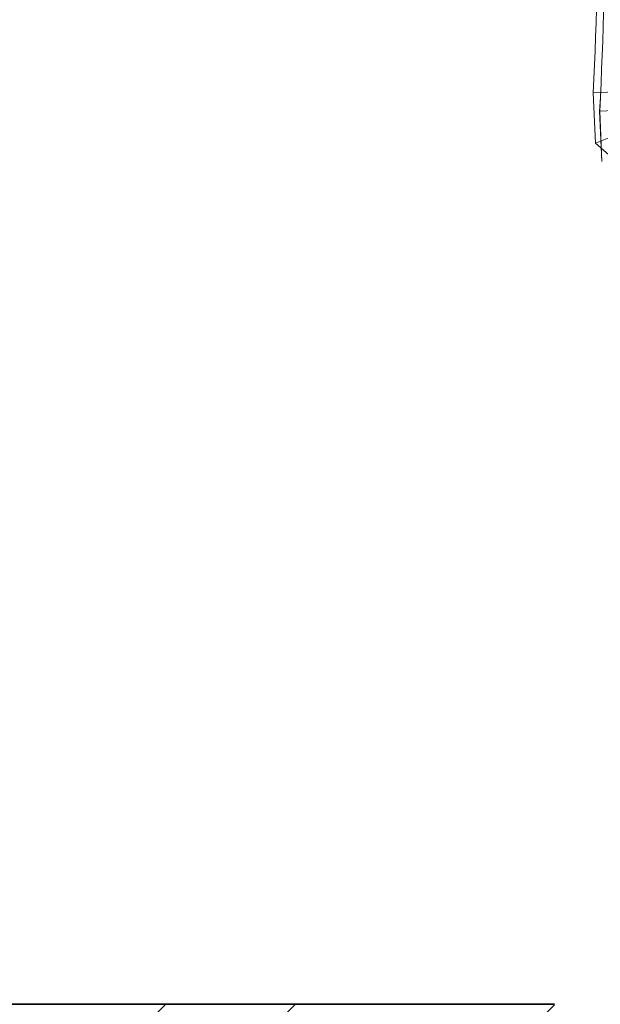
# Model space of a CAD drawing. Units: inches. Extents: x 1885 to 2748, y 783 to 2421.
# Tile 60 of 117: x 2029 to 2049, y 1886 to 1920. Entities that reach past the tile are written whole.
import ezdxf

# ---------------------------------------------------------------- set-up
doc = ezdxf.new("R2010")
doc.units = ezdxf.units.IN
doc.layers.add('A-FURN', color=8, linetype='Continuous', lineweight=13)
doc.layers.add('A-WALL', color=7, linetype='Continuous', lineweight=35)
doc.layers.add('A-WALL-PATT', color=85, linetype='Continuous', lineweight=13, true_color=0x58ba48)

# ---------------------------------------------------------------- blocks, each defined once
blk = doc.blocks.new('BED-DOUBLE')
for p, q in [((30.133, 53.174), (28.389, 53.095, 3.871)), ((30.133, 53.174), (28.389, 53.094, 3.871)), ((28.389, 53.095), (25.139, 49.389)), ((28.389, 53.094), (25.139, 49.389)), ((29.494, 52.946), (27.749, 52.866, 3.871)), ((29.494, 52.945), (27.75, 52.866, 3.871)), ((29.008, 51.558), (28.389, 53.095)), ((29.008, 51.557), (28.389, 53.094))]:
    blk.add_line(p, q)
for centre, radius, start, end in [((-6.013, 51.554), 36.183, 349.8763, 2.5657), ((-6.013, 51.554), 36.183, 349.8763, 2.5657), ((36.958, 182.493), 129.499, 266.97912, 273.83645), ((36.958, 182.493), 129.499, 266.97912, 273.83645), ((-6.653, 51.326), 36.183, 349.8763, 2.5657), ((-6.653, 51.326), 36.183, 349.8763, 2.5657), ((36.319, 182.265), 129.499, 266.97912, 273.83645), ((36.319, 182.264), 129.499, 266.97912, 273.83645)]:
    blk.add_arc(centre, radius, start, end)

msp = doc.modelspace()

# ---------------------------------------------------------------- hatches: boundary and pattern name
at = {"layer": 'A-WALL-PATT'}
h = msp.add_hatch(dxfattribs=at)
h.set_pattern_fill('ANSI32', color=256)
h.paths.add_polyline_path([(2007.772, 2318.006), (1980.774, 2318.006), (1980.774, 2281.215), (1985.274, 2281.215), (1985.274, 2313.506), (2007.772, 2313.506), (2007.772, 2315.756)])
h.paths.add_polyline_path([(2094.324, 2318.006), (2067.772, 2318.006), (2067.772, 2313.506), (2094.324, 2313.506), (2094.324, 2315.756)])
h.paths.add_polyline_path([(2131.367, 2315.756), (2131.367, 2318.006), (2131.189, 2318.006), (2112.609, 2318.006), (2112.609, 2313.506), (2117.274, 2313.506), (2117.274, 2255.201), (2121.774, 2255.201), (2121.774, 2313.506), (2131.367, 2313.506)])
h.paths.add_polyline_path([(2190.512, 2318.006), (2155.367, 2318.006), (2155.367, 2313.506), (2169.774, 2313.506), (2169.774, 2229.506), (2121.774, 2229.506), (2121.774, 2233.451), (2119.524, 2233.451), (2117.274, 2233.451), (2117.274, 2201.101), (2121.774, 2201.101), (2121.774, 2225.006), (2169.774, 2225.006), (2169.774, 2165.006), (2306.274, 2165.006), (2306.274, 2066.006), (2310.774, 2066.006), (2344.274, 2066.006), (2486.274, 2066.006), (2486.274, 1886.006), (2483.02, 1886.006), (2483.02, 1881.506), (2486.274, 1881.506), (2486.274, 1880.678), (2490.774, 1880.678), (2490.774, 2070.506), (2344.274, 2070.506), (2310.774, 2070.506), (2310.774, 2165.006), (2310.774, 2173.636), (2308.524, 2173.636), (2306.274, 2173.636), (2306.274, 2169.506), (2174.274, 2169.506), (2174.274, 2313.506), (2190.512, 2313.506), (2190.512, 2315.756)])
h.paths.add_polyline_path([(1985.274, 2221.215), (1980.774, 2221.215), (1980.774, 2165.006), (1992.774, 2165.006), (1992.774, 2141.927), (1997.274, 2141.927), (1997.274, 2165.006), (2117.274, 2165.006), (2117.274, 2163.126), (2121.774, 2163.126), (2121.774, 2172.734), (2119.524, 2172.734), (2117.274, 2172.734), (2117.274, 2169.506), (1985.274, 2169.506)])
h.paths.add_polyline_path([(1997.274, 2105.927), (1992.774, 2105.927), (1992.774, 2070.506), (2016.774, 2070.506), (2016.774, 2059.123), (2019.024, 2059.123), (2021.274, 2059.123), (2021.274, 2070.506), (2117.274, 2070.506), (2117.274, 2022.506), (2114.423, 2022.506), (2114.423, 2018.006), (2123.627, 2018.006), (2123.627, 2020.256), (2123.627, 2022.506), (2121.774, 2022.506), (2121.774, 2142.587), (2119.524, 2142.587), (2117.274, 2142.587), (2117.274, 2075.006), (1997.274, 2075.006)])
h.paths.add_polyline_path([(2092.029, 2020.256), (2092.029, 2022.506), (2021.274, 2022.506), (2021.274, 2035.123), (2016.774, 2035.123), (2016.774, 2018.006), (2016.774, 1978.784), (2021.274, 1978.784), (2021.274, 2018.006), (2092.029, 2018.006)])
h.paths.add_polyline_path([(2260.938, 2022.506), (2153.105, 2022.506), (2153.105, 2020.256), (2153.105, 2018.006), (2155.274, 2018.006), (2155.274, 1886.006), (2107.629, 1886.006), (2107.629, 1881.506), (2182.911, 1881.506), (2182.911, 1883.756), (2182.911, 1886.006), (2159.774, 1886.006), (2159.774, 2018.006), (2260.938, 2018.006), (2260.938, 2020.256)])
h.paths.add_polyline_path([(2047.629, 1883.756), (2047.629, 1886.006), (2021.274, 1886.006), (2021.274, 1918.784), (2019.024, 1918.784), (2016.774, 1918.784), (2016.774, 1881.506), (2047.629, 1881.506)])
h.paths.add_polyline_path([(2306.361, 1883.756), (2306.361, 1886.006), (2296.274, 1886.006), (2296.274, 1982.006), (2316.535, 1982.006), (2316.535, 1984.256), (2316.535, 1986.506), (2296.274, 1986.506), (2296.274, 2022.506), (2289.276, 2022.506), (2289.276, 2018.006), (2291.774, 2018.006), (2291.774, 1886.006), (2242.911, 1886.006), (2242.911, 1881.506), (2306.361, 1881.506)], flags=17)
h.paths.add_polyline_path([(1985.274, 1843.006), (2021.6, 1843.006), (2021.534, 1845.441), (2021.477, 1847.506), (1980.774, 1847.506), (1980.774, 1809.446), (1985.274, 1809.446)])
h.paths.add_polyline_path([(2131.482, 1845.256), (2131.482, 1847.506), (2081.534, 1847.506), (2081.534, 1843.006), (2117.274, 1843.006), (2117.274, 1784.147), (2119.524, 1784.147), (2121.774, 1784.147), (2121.774, 1843.006), (2131.482, 1843.006)])
h.paths.add_polyline_path([(2203.886, 1847.506), (2155.482, 1847.506), (2155.482, 1843.006), (2169.774, 1843.006), (2169.774, 1759.006), (2121.774, 1759.006), (2121.774, 1761.457), (2117.274, 1761.457), (2117.274, 1730.429), (2121.774, 1730.429), (2121.774, 1754.506), (2177.421, 1754.506), (2177.421, 1756.756), (2177.421, 1759.006), (2174.274, 1759.006), (2174.274, 1843.006), (2203.886, 1843.006)])
h.paths.add_polyline_path([(2335.554, 1845.256), (2335.554, 1847.506), (2239.886, 1847.506), (2239.886, 1843.006), (2306.274, 1843.006), (2306.274, 1759.006), (2199.486, 1759.006), (2199.486, 1754.506), (2310.774, 1754.506), (2310.774, 1843.006), (2335.554, 1843.006)])
h.paths.add_polyline_path([(2348.774, 2022.506), (2344.274, 2022.506), (2344.274, 1986.506), (2341.681, 1986.506), (2341.681, 1982.006), (2344.274, 1982.006), (2344.274, 1886.006), (2330.361, 1886.006), (2330.361, 1881.506), (2361.627, 1881.506), (2361.627, 1883.756), (2361.627, 1886.006), (2348.774, 1886.006)], flags=17)
h.paths.add_polyline_path([(2283.251, 2315.756), (2283.251, 2318.006), (2238.512, 2318.006), (2238.512, 2313.506), (2283.251, 2313.506)], flags=17)
h.paths.add_polyline_path([(2363.274, 2348.006), (2388.677, 2348.006), (2388.677, 2350.256), (2388.677, 2352.506), (2358.774, 2352.506), (2358.774, 2348.006), (2358.774, 2318.006), (2344.481, 2318.006), (2344.481, 2313.506), (2358.774, 2313.506), (2358.774, 2229.506), (2310.774, 2229.506), (2310.774, 2231.952), (2306.274, 2231.952), (2306.274, 2205.611), (2310.774, 2205.611), (2310.774, 2225.006), (2358.774, 2225.006), (2358.774, 2211.506), (2452.329, 2211.506), (2452.329, 2213.756), (2452.329, 2216.006), (2363.274, 2216.006), (2363.274, 2318.006)])
h.paths.add_polyline_path([(2310.774, 2313.506), (2320.481, 2313.506), (2320.481, 2315.756), (2320.481, 2318.006), (2302.728, 2318.006), (2302.728, 2313.506), (2306.274, 2313.506), (2306.274, 2251.076), (2310.774, 2251.076)], flags=17)
h.paths.add_polyline_path([(2490.774, 2352.506), (2486.274, 2352.506), (2448.677, 2352.506), (2448.677, 2348.006), (2486.274, 2348.006), (2486.274, 2318.006), (2486.274, 2216.006), (2481.78, 2216.006), (2481.78, 2211.506), (2486.274, 2211.506), (2486.274, 2165.006), (2493.289, 2165.006), (2493.289, 2167.256), (2493.289, 2169.506), (2490.774, 2169.506), (2490.774, 2313.506), (2494.429, 2313.506), (2494.429, 2318.006), (2490.774, 2318.006)])
h.paths.add_polyline_path([(2534.653, 2318.006), (2515.691, 2318.006), (2515.691, 2313.506), (2534.653, 2313.506), (2534.653, 2315.756)])
h.paths.add_polyline_path([(2618.274, 2318.006), (2594.653, 2318.006), (2594.653, 2313.506), (2613.774, 2313.506), (2613.774, 2281.706), (2618.274, 2281.706)])
h.paths.add_polyline_path([(2618.274, 2221.706), (2613.774, 2221.706), (2613.774, 2169.506), (2554.019, 2169.506), (2554.019, 2165.006), (2613.774, 2165.006), (2613.774, 2152.878), (2618.274, 2152.878)])
h.paths.add_polyline_path([(2618.274, 2128.878), (2616.024, 2128.878), (2613.774, 2128.878), (2613.774, 2117.006), (2529.774, 2117.006), (2529.774, 2165.006), (2532.848, 2165.006), (2532.848, 2169.506), (2522.867, 2169.506), (2522.867, 2165.006), (2525.274, 2165.006), (2525.274, 2117.006), (2525.274, 2112.506), (2525.274, 2108.576), (2529.774, 2108.576), (2529.774, 2112.506), (2613.774, 2112.506), (2613.774, 2080.19), (2618.274, 2080.19)])
h.paths.add_polyline_path([(2618.274, 2044.19), (2616.024, 2044.19), (2613.774, 2044.19), (2613.774, 2015.506), (2529.774, 2015.506), (2529.774, 2088.582), (2527.524, 2088.582), (2525.274, 2088.582), (2525.274, 2011.006), (2613.774, 2011.006), (2613.774, 1956.755), (2618.274, 1956.755)])
h.paths.add_polyline_path([(2618.274, 1881.506), (2618.274, 1896.755), (2613.774, 1896.755), (2613.774, 1881.506), (2613.774, 1847.506), (2592.715, 1847.506), (2592.715, 1843.006), (2613.774, 1843.006), (2613.774, 1765.006), (2613.774, 1760.506), (2609.621, 1760.506), (2609.621, 1756.006), (2613.774, 1756.006), (2613.774, 1660.006), (2608.544, 1660.006), (2608.544, 1655.506), (2613.774, 1655.506), (2613.774, 1508.158), (2618.274, 1508.158)])
h.paths.add_polyline_path([(2565.774, 1843.006), (2568.997, 1843.006), (2568.997, 1847.506), (2490.774, 1847.506), (2490.774, 1849.7), (2488.524, 1849.7), (2486.274, 1849.7), (2486.274, 1847.506), (2477.274, 1847.506), (2477.274, 1838.506), (2477.274, 1821.493), (2486.274, 1821.493), (2486.274, 1838.506), (2561.274, 1838.506), (2561.274, 1765.006), (2486.274, 1765.006), (2486.274, 1786.157), (2477.274, 1786.157), (2477.274, 1765.006), (2477.274, 1756.006), (2486.274, 1756.006), (2565.774, 1756.006), (2585.621, 1756.006), (2585.621, 1758.256), (2585.621, 1760.506), (2565.774, 1760.506), (2565.774, 1765.006)])
h.paths.add_polyline_path([(2486.274, 1651.006), (2561.274, 1651.006), (2561.274, 1567.006), (2486.274, 1567.006), (2486.274, 1591.321), (2477.274, 1591.321), (2477.274, 1567.006), (2477.274, 1558.006), (2477.274, 1555.439), (2481.774, 1555.439), (2481.774, 1558.006), (2568.653, 1558.006), (2568.653, 1560.256), (2568.653, 1562.506), (2565.774, 1562.506), (2565.774, 1655.506), (2584.544, 1655.506), (2584.544, 1657.756), (2584.544, 1660.006), (2565.774, 1660.006), (2486.274, 1660.006), (2477.274, 1660.006), (2477.274, 1651.006), (2477.274, 1632.989), (2486.274, 1632.989)])
h.paths.add_polyline_path([(2449.967, 1883.756), (2449.967, 1886.006), (2421.627, 1886.006), (2421.627, 1881.506), (2449.967, 1881.506)], flags=17)
h.paths.add_polyline_path([(2447.274, 1847.506), (2395.554, 1847.506), (2395.554, 1843.006), (2442.774, 1843.006), (2442.774, 1809.27), (2447.274, 1809.27)])
h.paths.add_polyline_path([(1985.274, 1749.446), (1980.774, 1749.446), (1980.774, 1694.504), (1985.274, 1694.504), (1985.274, 1694.506), (1986.897, 1694.506), (1986.897, 1697.78), (1986.897, 1699.006), (1985.274, 1699.006)])
h.paths.add_polyline_path([(2152.774, 1699.006), (2121.774, 1699.006), (2121.774, 1703.668), (2119.524, 1703.668), (2117.274, 1703.668), (2117.274, 1699.006), (2009.219, 1699.006), (2009.219, 1694.506), (2148.274, 1694.506), (2148.274, 1692.631), (2152.774, 1692.631)])
h.paths.add_polyline_path([(2016.274, 1694.506), (2011.774, 1694.506), (2011.774, 1558.006), (2040.806, 1558.006), (2040.806, 1560.256), (2040.806, 1562.506), (2016.274, 1562.506)])
h.paths.add_polyline_path([(2152.774, 1663.017), (2150.524, 1663.017), (2148.274, 1663.017), (2148.274, 1562.506), (2100.806, 1562.506), (2100.806, 1558.006), (2165.119, 1558.006), (2165.119, 1560.256), (2165.119, 1562.506), (2152.774, 1562.506), (2152.774, 1610.506), (2224.774, 1610.506), (2224.774, 1607.99), (2229.274, 1607.99), (2229.274, 1615.006), (2152.774, 1615.006)])
h.paths.add_polyline_path([(2238.613, 1560.256), (2238.613, 1562.506), (2229.274, 1562.506), (2229.274, 1588.756), (2227.024, 1588.763), (2224.774, 1588.771), (2224.774, 1562.506), (2189.119, 1562.506), (2189.119, 1558.006), (2238.613, 1558.006)])
h.paths.add_polyline_path([(2336.024, 1560.256), (2336.024, 1562.506), (2310.774, 1562.506), (2310.774, 1656.347), (2308.524, 1656.347), (2306.274, 1656.347), (2306.274, 1562.506), (2286.613, 1562.506), (2286.613, 1558.006), (2336.024, 1558.006)])
h.paths.add_polyline_path([(2447.274, 1690.968), (2445.024, 1690.968), (2442.774, 1690.968), (2442.774, 1687.006), (2306.274, 1687.006), (2306.274, 1680.75), (2310.774, 1680.75), (2310.774, 1682.506), (2442.774, 1682.506), (2442.774, 1562.506), (2396.024, 1562.506), (2396.024, 1558.006), (2447.274, 1558.006)])
h.paths.add_polyline_path([(2447.274, 1749.27), (2445.024, 1749.27), (2442.774, 1749.27), (2442.774, 1717.232), (2447.274, 1717.232)])
h.paths.add_polyline_path([(2044.674, 1521.756), (2044.674, 1524.006), (2007.274, 1524.006), (2007.274, 1503.49), (2009.524, 1503.49), (2011.774, 1503.49), (2011.774, 1519.506), (2044.674, 1519.506)])
h.paths.add_polyline_path([(2177.969, 1521.756), (2177.969, 1524.006), (2104.674, 1524.006), (2104.674, 1519.506), (2145.774, 1519.506), (2145.774, 1387.506), (2143.37, 1387.506), (2143.37, 1383.006), (2251.585, 1383.006), (2251.585, 1385.256), (2251.585, 1387.506), (2150.274, 1387.506), (2150.274, 1519.506), (2177.969, 1519.506)])
h.paths.add_polyline_path([(2298.704, 1524.006), (2237.969, 1524.006), (2237.969, 1519.506), (2282.274, 1519.506), (2282.274, 1387.506), (2279.683, 1387.506), (2279.683, 1383.006), (2286.774, 1383.006), (2286.774, 1419.006), (2312.451, 1419.006), (2312.451, 1421.256), (2312.451, 1423.506), (2286.774, 1423.506), (2286.774, 1519.506), (2298.704, 1519.506), (2298.704, 1521.722)], flags=17)
h.paths.add_polyline_path([(2361.897, 1521.756), (2361.897, 1524.006), (2322.704, 1524.006), (2322.704, 1519.506), (2334.774, 1519.506), (2334.774, 1423.506), (2331.93, 1423.506), (2331.93, 1419.006), (2334.774, 1419.006), (2334.774, 1387.506), (2334.774, 1383.228), (2339.274, 1383.228), (2339.274, 1387.506), (2339.274, 1519.506), (2361.897, 1519.506)], flags=17)
h.paths.add_polyline_path([(2447.274, 1521.756), (2447.274, 1524.006), (2421.897, 1524.006), (2421.897, 1519.506), (2447.274, 1519.506)], flags=17)
h.paths.add_polyline_path([(2481.774, 1529.6), (2479.524, 1529.6), (2477.274, 1529.6), (2477.274, 1524.006), (2474.489, 1524.006), (2474.489, 1519.506), (2477.274, 1519.506), (2477.274, 1334.506), (2296.774, 1334.506), (2296.774, 1240.506), (2160.274, 1240.506), (2160.274, 1180.506), (2112.274, 1180.506), (2112.274, 1207.692), (2110.024, 1207.692), (2107.774, 1207.692), (2107.774, 1171.609), (2112.274, 1171.609), (2112.274, 1176.006), (2160.274, 1176.006), (2160.274, 1092.006), (2144.221, 1092.006), (2144.221, 1087.506), (2189.497, 1087.506), (2189.497, 1089.756), (2189.497, 1092.006), (2164.774, 1092.006), (2164.774, 1236.006), (2296.774, 1236.006), (2296.774, 1231.912), (2301.274, 1231.912), (2301.274, 1330.006), (2481.774, 1330.006), (2481.774, 1387.506)])
h.paths.add_polyline_path([(2618.274, 1448.158), (2613.774, 1448.158), (2613.774, 1382.506), (2529.774, 1382.506), (2525.274, 1382.506), (2525.274, 1307.062), (2529.774, 1307.062), (2529.774, 1378.006), (2613.774, 1378.006), (2613.774, 1354.988), (2618.274, 1354.988)])
h.paths.add_polyline_path([(2618.274, 1318.988), (2613.774, 1318.988), (2613.774, 1281.006), (2529.774, 1281.006), (2529.774, 1283.786), (2527.524, 1283.786), (2525.274, 1283.786), (2525.274, 1228.506), (2516.794, 1228.506), (2516.794, 1224.006), (2533.484, 1224.006), (2533.484, 1226.256), (2533.484, 1228.506), (2529.774, 1228.506), (2529.774, 1276.506), (2613.774, 1276.506), (2613.774, 1266.02), (2618.274, 1266.02)])
h.paths.add_polyline_path([(2618.274, 1134.964), (2613.774, 1134.964), (2613.774, 1092.006), (2594.545, 1092.006), (2594.545, 1087.506), (2618.274, 1087.506)])
h.paths.add_polyline_path([(2534.545, 1092.006), (2509.765, 1092.006), (2509.765, 1087.506), (2534.545, 1087.506), (2534.545, 1089.756)])
h.paths.add_polyline_path([(2481.274, 1224.006), (2484.117, 1224.006), (2484.117, 1226.256), (2484.117, 1228.506), (2476.774, 1228.506), (2476.774, 1198.506), (2471.61, 1198.506), (2471.61, 1194.006), (2476.774, 1194.006), (2476.774, 1062.006), (2436.894, 1062.006), (2436.894, 1057.506), (2476.774, 1057.506), (2481.274, 1057.506), (2481.274, 1062.006), (2481.274, 1087.506), (2485.354, 1087.506), (2485.354, 1089.756), (2485.354, 1092.006), (2481.274, 1092.006), (2481.274, 1117.506)])
h.paths.add_polyline_path([(2439.898, 1198.506), (2349.274, 1198.506), (2349.274, 1194.006), (2349.274, 1180.506), (2301.274, 1180.506), (2301.274, 1201.896), (2299.024, 1201.896), (2296.774, 1201.896), (2296.774, 1172.335), (2299.024, 1172.335), (2301.274, 1172.335), (2301.274, 1176.006), (2349.274, 1176.006), (2349.274, 1092.006), (2334.452, 1092.006), (2334.452, 1087.506), (2349.274, 1087.506), (2349.274, 1057.506), (2353.774, 1057.506), (2376.894, 1057.506), (2376.894, 1059.756), (2376.894, 1062.006), (2353.774, 1062.006), (2353.774, 1087.506), (2353.774, 1180.506), (2353.774, 1194.006), (2439.898, 1194.006), (2439.898, 1196.256)])
h.paths.add_polyline_path([(2270.596, 1089.756), (2270.596, 1092.006), (2249.497, 1092.006), (2249.497, 1087.506), (2270.596, 1087.506)], flags=17)
h.paths.add_polyline_path([(2310.452, 1092.006), (2301.274, 1092.006), (2301.274, 1153.292), (2296.774, 1153.292), (2296.774, 1092.006), (2293.786, 1092.006), (2293.786, 1087.506), (2310.452, 1087.506), (2310.452, 1089.756)], flags=17)
h.paths.add_polyline_path([(2112.274, 1150.328), (2110.024, 1150.328), (2107.774, 1150.328), (2107.774, 1092.006), (2104.465, 1092.006), (2104.465, 1087.506), (2120.221, 1087.506), (2120.221, 1089.756), (2120.221, 1092.006), (2112.274, 1092.006)])
h.paths.add_polyline_path([(2082.172, 1092.006), (2058.144, 1092.006), (2058.144, 1087.506), (2082.172, 1087.506), (2082.172, 1089.756)])
h.paths.add_polyline_path([(1975.774, 1145.638), (1971.274, 1145.638), (1971.274, 1087.506), (1980.774, 1087.506), (1998.144, 1087.506), (1998.144, 1089.756), (1998.144, 1092.006), (1985.274, 1092.006), (1975.774, 1092.006)])
h.paths.add_polyline_path([(2112.274, 1244.385), (2110.024, 1244.385), (2107.774, 1244.385), (2107.774, 1240.506), (1992.274, 1240.506), (1992.274, 1271.008), (1987.774, 1271.008), (1987.774, 1240.506), (1980.774, 1240.506), (1975.774, 1240.506), (1971.274, 1240.506), (1971.274, 1205.638), (1975.774, 1205.638), (1975.774, 1236.006), (2107.774, 1236.006), (2107.774, 1233.444), (2112.274, 1233.444), (2112.274, 1236.006)])
h.paths.add_polyline_path([(2112.274, 1383.006), (2114.783, 1383.006), (2114.783, 1385.256), (2114.783, 1387.506), (2102.476, 1387.506), (2102.476, 1383.006), (2107.774, 1383.006), (2107.774, 1335.006), (2011.774, 1335.006), (2011.774, 1349.939), (2007.274, 1349.939), (2007.274, 1335.006), (1987.774, 1335.006), (1987.774, 1330.506), (1987.774, 1307.008), (1992.274, 1307.008), (1992.274, 1330.506), (2007.274, 1330.506), (2107.774, 1330.506), (2107.774, 1264.711), (2112.274, 1264.711)])
h.paths.add_polyline_path([(2077.857, 1387.506), (2011.774, 1387.506), (2011.774, 1390.036), (2009.524, 1390.036), (2007.274, 1390.036), (2007.274, 1373.939), (2011.774, 1373.939), (2011.774, 1383.006), (2077.857, 1383.006)])
h.paths.add_polyline_path([(2011.774, 1443.49), (2007.274, 1443.49), (2007.274, 1410.248), (2011.774, 1410.248)])

# ---------------------------------------------------------------- linework, layer by layer
at = {"layer": 'A-WALL'}
msp.add_line((2021.274, 1886.006), (2047.629, 1886.006), dxfattribs=at)

# ---------------------------------------------------------------- block references
at = {"layer": 'A-FURN', "rotation": 89.9999998331857}
msp.add_blockref('BED-DOUBLE', (2102.136, 1887.416), dxfattribs=at)

doc.saveas('drawing.dxf')
